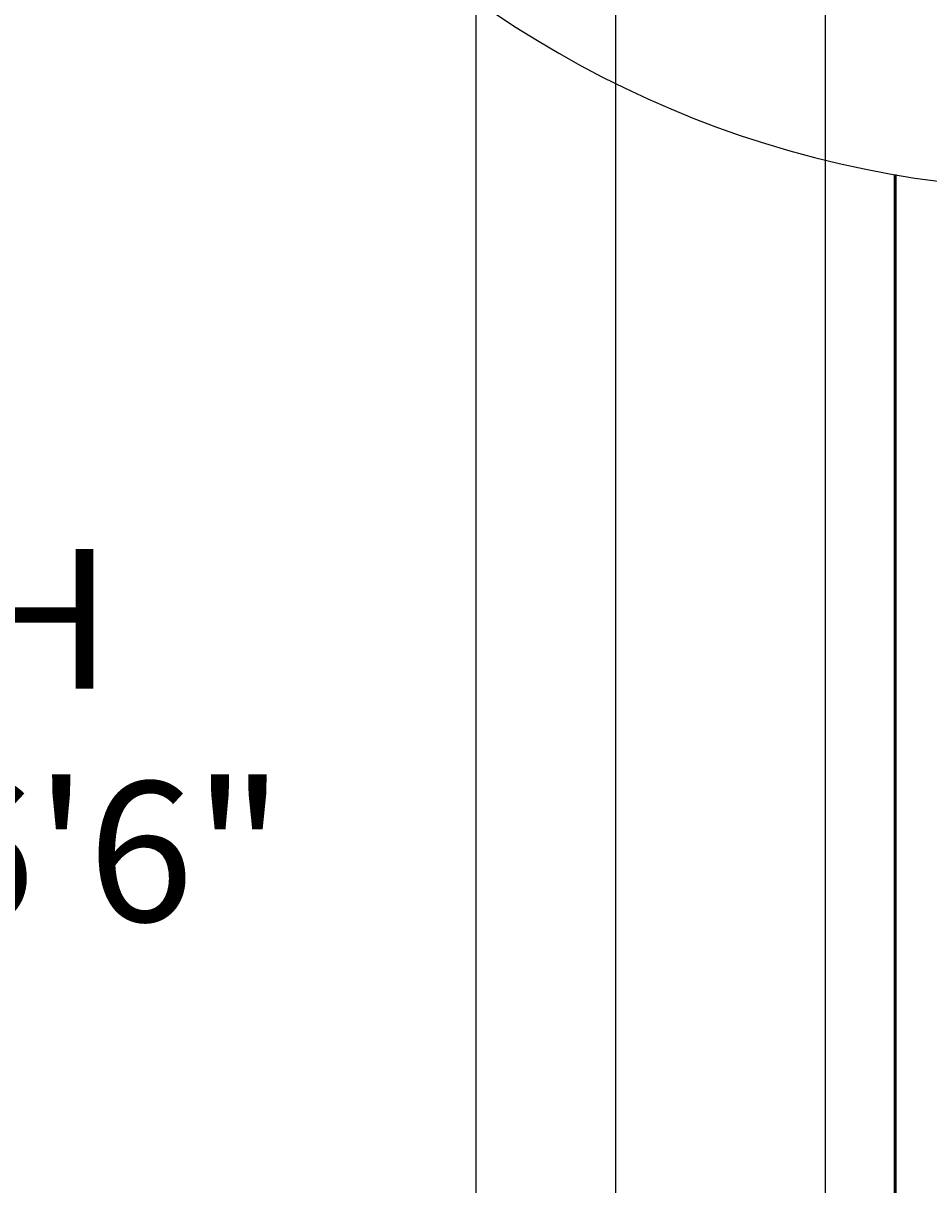
# Model space of a CAD drawing. Units: inches. Extents: x 37 to 824, y -700 to 234.
# Tile 46 of 77: x 193 to 219, y 17 to 50. Entities that reach past the tile are written whole.
import ezdxf

# ---------------------------------------------------------------- set-up
doc = ezdxf.new("R2010")
doc.units = ezdxf.units.IN
doc.header["$MEASUREMENT"] = 0
for name, color, linetype, lineweight in [('A-ANNO-DIMS', 2, 'Continuous', 18), ('A-AREA-IDEN', 3, 'Continuous', 18), ('A-DOOR', 4, 'Continuous', 25), ('A-WALL', 2, 'Continuous', 50)]:
    doc.layers.add(name, color=color, linetype=linetype, lineweight=lineweight)
doc.styles.get("Standard").update_dxf_attribs({"font": 'arial.ttf'})
doc.dimstyles.get("Standard").update_dxf_attribs({"dimtxt": 0.18, "dimasz": 0.18, "dimexe": 0.18, "dimexo": 0.0625, "dimgap": 0.09, "dimtad": 0, "dimtih": 1, "dimtoh": 1, "dimdec": 1, "dimzin": 0, "dimdsep": 46, "dimlunit": 4, "dimtxsty": 'Standard', "dimcen": 0.09, "dimadec": 0, "dimazin": 0, "dimtfac": 1, "dimtdec": 1, "dimtofl": 0, "dimtmove": 0, "dimatfit": 3, "dimfxl": 1, "dimtolj": 1, "dimtzin": 0, "dimarcsym": 0})

# ---------------------------------------------------------------- blocks, each defined once
blk = doc.blocks.new('*U6')
for p, q in [((-750, 0), (-750, -100)), ((0, 0), (0, -100))]:
    blk.add_line(p, q)
blk.add_lwpolyline([(0, 0), (0, 750), (-43.75, 750), (-43.75, 0)], close=True)
blk.add_arc((0, 0), 750, 90, 180)
blk = doc.blocks.new('*D84')
at = {"layer": 'A-ANNO-DIMS', "color": 0, "lineweight": -2, "ltscale": 0.5, "transparency": 16777216}
for p, q in [((170.077, -265.847), (170.077, 234.17)), ((210.077, -265.847), (210.077, 234.17)), ((170.257, 233.99), (189.748, 233.99)), ((209.897, 233.99), (190.406, 233.99))]:
    blk.add_line(p, q, dxfattribs=at)
at = {"layer": 'A-ANNO-DIMS', "color": 0, "ltscale": 0.5, "transparency": 16777216}
for points in [[(170.257, 234.02), (170.257, 233.96), (170.077, 233.99)], [(209.897, 234.02), (209.897, 233.96), (210.077, 233.99)]]:
    blk.add_solid(points, dxfattribs=at)
at = {"layer": 'Defpoints', "color": 0, "ltscale": 0.5, "transparency": 16777216}
for p in [(210.077, 233.99), (170.077, -265.91), (210.077, -265.91)]:
    blk.add_point(p, dxfattribs=at)
at = {"layer": 'A-ANNO-DIMS', "color": 0, "ltscale": 0.5, "transparency": 16777216, "insert": (190.077, 233.99), "char_height": 0.18, "attachment_point": 5}
blk.add_mtext('\\A1;3\'-4"', dxfattribs=at)
blk = doc.blocks.new('*D85')
at = {"layer": 'A-ANNO-DIMS', "color": 0, "lineweight": -2, "ltscale": 0.5, "transparency": 16777216}
for p, q in [((170.077, -356.847), (170.077, 234.17)), ((206.077, -356.847), (206.077, 234.17)), ((170.257, 233.99), (187.748, 233.99)), ((205.897, 233.99), (188.406, 233.99))]:
    blk.add_line(p, q, dxfattribs=at)
at = {"layer": 'A-ANNO-DIMS', "color": 0, "ltscale": 0.5, "transparency": 16777216}
for points in [[(170.257, 234.02), (170.257, 233.96), (170.077, 233.99)], [(205.897, 234.02), (205.897, 233.96), (206.077, 233.99)]]:
    blk.add_solid(points, dxfattribs=at)
at = {"layer": 'Defpoints', "color": 0, "ltscale": 0.5, "transparency": 16777216}
for p in [(206.077, 233.99), (170.077, -356.91), (206.077, -356.91)]:
    blk.add_point(p, dxfattribs=at)
at = {"layer": 'A-ANNO-DIMS', "color": 0, "ltscale": 0.5, "transparency": 16777216, "insert": (188.077, 233.99), "char_height": 0.18, "attachment_point": 5}
blk.add_mtext('\\A1;3\'-0"', dxfattribs=at)
blk = doc.blocks.new('*D86')
at = {"layer": 'A-ANNO-DIMS', "color": 0, "lineweight": -2, "ltscale": 0.5, "transparency": 16777216}
for p, q in [((206.077, -356.847), (206.077, 234.17)), ((216.077, -356.847), (216.077, 234.17)), ((206.257, 233.99), (210.678, 233.99)), ((215.897, 233.99), (211.476, 233.99))]:
    blk.add_line(p, q, dxfattribs=at)
at = {"layer": 'A-ANNO-DIMS', "color": 0, "ltscale": 0.5, "transparency": 16777216}
for points in [[(206.257, 234.02), (206.257, 233.96), (206.077, 233.99)], [(215.897, 234.02), (215.897, 233.96), (216.077, 233.99)]]:
    blk.add_solid(points, dxfattribs=at)
at = {"layer": 'Defpoints', "color": 0, "ltscale": 0.5, "transparency": 16777216}
for p in [(216.077, 233.99), (206.077, -356.91), (216.077, -356.91)]:
    blk.add_point(p, dxfattribs=at)
at = {"layer": 'A-ANNO-DIMS', "color": 0, "ltscale": 0.5, "transparency": 16777216, "insert": (211.077, 233.99), "char_height": 0.18, "attachment_point": 5}
blk.add_mtext('\\A1;0\'-10"', dxfattribs=at)
blk = doc.blocks.new('*D87')
at = {"layer": 'A-ANNO-DIMS', "color": 0, "lineweight": -2, "ltscale": 0.5, "transparency": 16777216}
for p, q in [((216.077, -356.847), (216.077, 234.17)), ((296.077, -356.847), (296.077, 234.17)), ((216.257, 233.99), (255.747, 233.99)), ((295.897, 233.99), (256.407, 233.99))]:
    blk.add_line(p, q, dxfattribs=at)
at = {"layer": 'A-ANNO-DIMS', "color": 0, "ltscale": 0.5, "transparency": 16777216}
for points in [[(216.257, 234.02), (216.257, 233.96), (216.077, 233.99)], [(295.897, 234.02), (295.897, 233.96), (296.077, 233.99)]]:
    blk.add_solid(points, dxfattribs=at)
at = {"layer": 'Defpoints', "color": 0, "ltscale": 0.5, "transparency": 16777216}
for p in [(296.077, 233.99), (216.077, -356.91), (296.077, -356.91)]:
    blk.add_point(p, dxfattribs=at)
at = {"layer": 'A-ANNO-DIMS', "color": 0, "ltscale": 0.5, "transparency": 16777216, "insert": (256.077, 233.99), "char_height": 0.18, "attachment_point": 5}
blk.add_mtext('\\A1;6\'-8"', dxfattribs=at)

msp = doc.modelspace()

# ---------------------------------------------------------------- linework, layer by layer
at = {"layer": 'A-WALL'}
msp.add_line((218.077, -2.91), (218.077, 46), dxfattribs=at)

# ---------------------------------------------------------------- block references
at = {"layer": 'A-DOOR', "xscale": 0.0393700787401575, "yscale": 0.0393700787401575, "zscale": 0.0393700787401575, "rotation": 90}
msp.add_blockref('*U6', (223.14, 75.09), dxfattribs=at)

# ---------------------------------------------------------------- texts
at = {"layer": 'A-AREA-IDEN', "insert": (176.627, 35.284), "char_height": 4, "attachment_point": 1}
msp.add_mtext_dynamic_manual_height_columns('    BATH\\P   4\' X 6\'6"', width=88.32168, gutter_width=1, heights=[0], dxfattribs=at)

# ---------------------------------------------------------------- dimensions: what is measured, and where the dimension line sits
at = {"layer": 'A-ANNO-DIMS', "ltscale": 0.5}
for base, p1, p2, picture, middle in [((210.077, 233.99), (170.077, -265.91), (210.077, -265.91), '*D84', (190.077, 233.99)), ((206.077, 233.99), (170.077, -356.91), (206.077, -356.91), '*D85', (188.077, 233.99)), ((216.077, 233.99), (206.077, -356.91), (216.077, -356.91), '*D86', (211.077, 233.99)), ((296.077, 233.99), (216.077, -356.91), (296.077, -356.91), '*D87', (256.077, 233.99))]:
    dim = msp.add_linear_dim(base=base, p1=p1, p2=p2, dimstyle='Standard', override={"dimdec": 1, "dimlfac": 1, "dimrnd": 0, "dimzin": 1, "dimdsep": 46, "dimlunit": 4, "dimfrac": 2}, dxfattribs=at)
    dim.commit()
    dim.dimension.update_dxf_attribs({"geometry": picture, "text_midpoint": middle})

doc.saveas('drawing.dxf')
